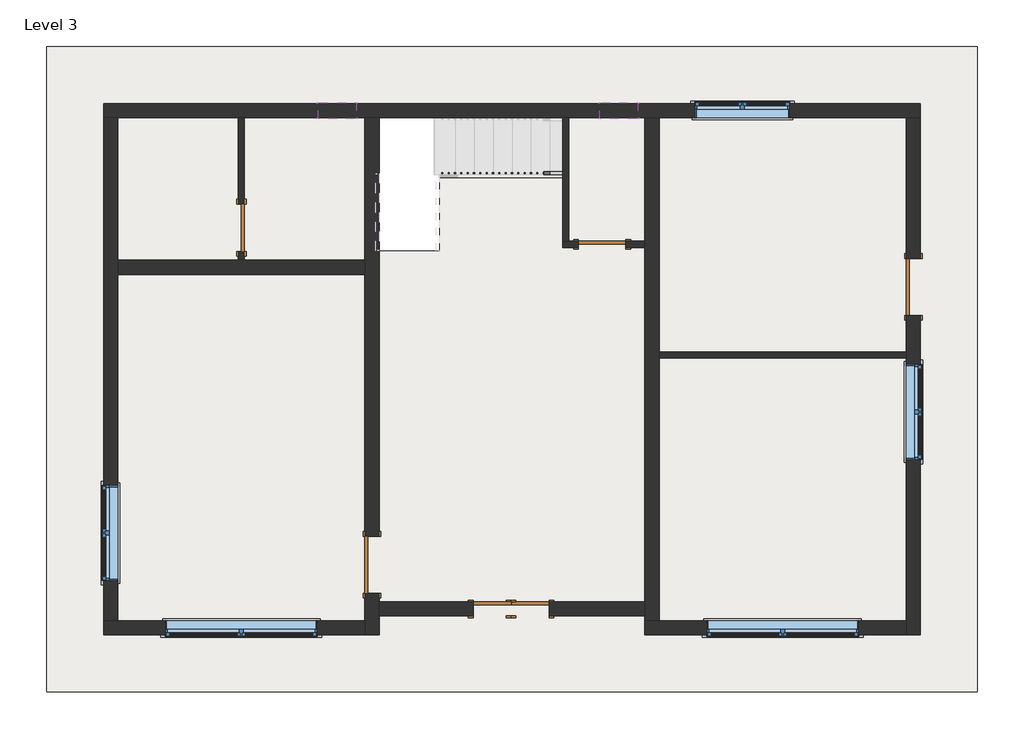
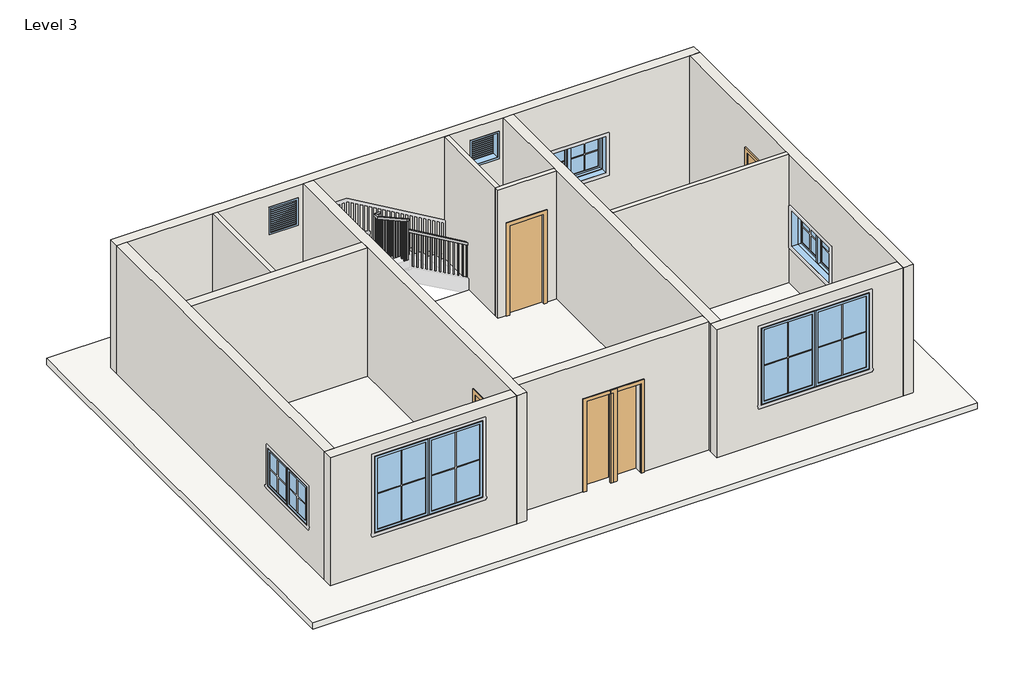
# One storey, part 1 of 2: 13 walls, 7 windows, 6 doors, 1 railing, 1 roof.
"""IFC4 building model written with IfcOpenShell, lengths in millimetres."""

from ifc_helpers import new_model, si_unit, frame, origin, place, context, project, spatial, polyline, outline, extrude, faceted_brep, transform, mapped, element, save
from components import single_flush_door_2_4a3212df, single_flush_door_2_0d3b4037, door_270f2424, door_aa9e95e7, single_flush_door_3_a90ba1ad, window_casement_double_c1d95f0f, window_casement_double_9ae172a2, window_f2d8fef0

model = new_model("IFC4")

# Units and contexts
model_context = context("Model", 3, world=origin())
ifc_project = project(units=[si_unit("LENGTHUNIT", "METRE", prefix="MILLI")], contexts=[model_context])

# Site, building, storey
site = spatial("IfcSite", under=ifc_project)
building = spatial("IfcBuilding", under=site)
storey = spatial("IfcBuildingStorey", under=building, Name="Level 3", Elevation=6248.4)

# Doors
placement = place(None, origin())
single_flush_door_2_shape = single_flush_door_2_4a3212df(model_context)
element("IfcDoor", 1, ObjectType="Single-Flush : DOOR 2'", at=placement, inside=storey, context=model_context, shape_type="MappedRepresentation", body=[
    mapped(single_flush_door_2_shape, transform((-1572.7415084, -2604.3618005, 6248.4), x_axis=(-1.0, 0.0, 0.0), y_axis=(0.0, -1.0, 0.0), z_axis=(0.0, 0.0, 1.0))),
])
single_flush_door_2_2_shape = single_flush_door_2_0d3b4037(model_context)
element("IfcDoor", 2, ObjectType="Single-Flush : DOOR 2'", at=placement, inside=storey, context=model_context, shape_type="MappedRepresentation", body=[
    mapped(single_flush_door_2_2_shape, transform((-963.1415084, -2604.3618005, 6248.4), x_axis=(1.0, 0.0, 0.0), y_axis=(0.0, 1.0, 0.0), z_axis=(0.0, 0.0, 1.0))),
])
door_shape = door_270f2424(model_context)
element("IfcDoor", 3, ObjectType="Single-Flush : DOOR 2'6\"", at=placement, inside=storey, context=model_context, shape_type="MappedRepresentation", body=[
    mapped(door_shape, transform((-5598.6415084, 3517.0381995, 6248.4), x_axis=(0.0, -1.0, 0.0), y_axis=(1.0, 0.0, 0.0), z_axis=(0.0, 0.0, 1.0))),
])
door_2_shape = door_aa9e95e7(model_context)
element("IfcDoor", 4, ObjectType="Single-Flush : DOOR 2'6\"", at=placement, inside=storey, context=model_context, shape_type="MappedRepresentation", body=[
    mapped(door_2_shape, transform((192.5584916, 3250.3381995, 6248.4), x_axis=(-1.0, 0.0, 0.0), y_axis=(0.0, -1.0, 0.0), z_axis=(0.0, 0.0, 1.0))),
])
single_flush_door_3_shape = single_flush_door_3_a90ba1ad(model_context)
element("IfcDoor", 5, ObjectType="Single-Flush : DOOR 3'", at=placement, inside=storey, context=model_context, shape_type="MappedRepresentation", body=[
    mapped(single_flush_door_3_shape, transform((-3503.1415084, -1893.1618005, 6248.4), x_axis=(0.0, -1.0, 0.0), y_axis=(1.0, 0.0, 0.0), z_axis=(0.0, 0.0, 1.0))),
])
element("IfcDoor", 6, ObjectType="Single-Flush : DOOR 3'", at=placement, inside=storey, context=model_context, shape_type="MappedRepresentation", body=[
    mapped(single_flush_door_3_shape, transform((5183.6584916, 2564.5381995, 6248.4), x_axis=(0.0, -1.0, 0.0), y_axis=(1.0, 0.0, 0.0), z_axis=(0.0, 0.0, 1.0))),
])

# Railing
element("IfcRailing", 7, ObjectType="Handrail - Rectangular", at=placement, inside=storey, context=model_context, shape_type="SolidModel", body=[
    faceted_brep([(-442.4415084, 4368.3146777, 7332.1333333), (-442.4415084, 4368.3146777, 7273.3219871), (-442.4415084, 4419.1146777, 7273.3219871), (-442.4415084, 4419.1146777, 7332.1333333), (-2398.2415084, 4368.3146777, 8473.0166667), (-2449.0415084, 4368.3146777, 8443.8386538), (-2449.0415084, 4419.1146777, 8443.8386538), (-2398.2415084, 4419.1146777, 8473.0166667), (-2398.2415084, 4368.3146777, 8729.1202697), (-2449.0415084, 4368.3146777, 8678.3202697), (-2449.0415084, 4419.1146777, 8678.3202697), (-2398.2415084, 4419.1146777, 8729.1202697), (-2474.4415084, 4368.3146777, 8729.1202697), (-2474.4415084, 4368.3146777, 8678.3202697), (-2525.2415084, 4419.1146777, 8678.3202697), (-2525.2415084, 4419.1146777, 8729.1202697), (-2474.4415084, 4292.1146777, 8729.1202697), (-2474.4415084, 4278.9546266, 8678.3202697), (-2525.2415084, 4278.9546266, 8678.3202697), (-2525.2415084, 4292.1146777, 8729.1202697), (-2474.4415084, 3148.7383287, 9364.1333333), (-2525.2415084, 3148.7383287, 9364.1333333), (-2525.2415084, 3148.7383287, 9306.02445), (-2474.4415084, 3148.7383287, 9306.02445)], [[[0, 1, 2, 3]], [[1, 0, 4, 5]], [[2, 1, 5, 6]], [[3, 2, 6, 7]], [[0, 3, 7, 4]], [[5, 4, 8, 9]], [[6, 5, 9, 10]], [[7, 6, 10, 11]], [[4, 7, 11, 8]], [[9, 8, 12, 13]], [[10, 9, 13, 14]], [[11, 10, 14, 15]], [[8, 11, 15, 12]], [[13, 12, 16, 17]], [[14, 13, 17, 18]], [[15, 14, 18, 19]], [[12, 15, 19, 16]], [[20, 21, 22, 23]], [[17, 16, 20, 23]], [[18, 17, 23, 22]], [[19, 18, 22, 21]], [[16, 19, 21, 20]]]),
    extrude(outline(polyline([(3184.0396777, 9286.5754052), (3184.0396777, 8280.4), (3164.9896777, 8280.4), (3164.9896777, 9297.1554726), (3184.0396777, 9286.5754052)])), frame((-2509.3665084, 0.0, 0.0), z_axis=(1.0, 0.0, 0.0), x_axis=(0.0, 1.0, 0.0)), (0.0, 0.0, 1.0), 19.05),
    extrude(outline(polyline([(3285.6396777, 9230.1483789), (3285.6396777, 8280.4), (3266.5896777, 8280.4), (3266.5896777, 9240.7284463), (3285.6396777, 9230.1483789)])), frame((-2509.3665084, 0.0, 0.0), z_axis=(1.0, 0.0, 0.0), x_axis=(0.0, 1.0, 0.0)), (0.0, 0.0, 1.0), 19.05),
    extrude(outline(polyline([(3387.2396777, 9173.7213526), (3387.2396777, 8280.4), (3368.1896777, 8280.4), (3368.1896777, 9184.3014201), (3387.2396777, 9173.7213526)])), frame((-2509.3665084, 0.0, 0.0), z_axis=(1.0, 0.0, 0.0), x_axis=(0.0, 1.0, 0.0)), (0.0, 0.0, 1.0), 19.05),
    extrude(outline(polyline([(3488.8396777, 9117.2420718), (3488.8396777, 8111.0666667), (3469.7896777, 8111.0666667), (3469.7896777, 9127.8221392), (3488.8396777, 9117.2420718)])), frame((-2509.3665084, 0.0, 0.0), z_axis=(1.0, 0.0, 0.0), x_axis=(0.0, 1.0, 0.0)), (0.0, 0.0, 1.0), 19.05),
    extrude(outline(polyline([(3590.4396777, 9060.8150456), (3590.4396777, 8111.0666667), (3571.3896777, 8111.0666667), (3571.3896777, 9071.395113), (3590.4396777, 9060.8150456)])), frame((-2509.3665084, 0.0, 0.0), z_axis=(1.0, 0.0, 0.0), x_axis=(0.0, 1.0, 0.0)), (0.0, 0.0, 1.0), 19.05),
    extrude(outline(polyline([(3692.0396777, 9004.3880193), (3692.0396777, 8111.0666667), (3672.9896777, 8111.0666667), (3672.9896777, 9014.9680867), (3692.0396777, 9004.3880193)])), frame((-2509.3665084, 0.0, 0.0), z_axis=(1.0, 0.0, 0.0), x_axis=(0.0, 1.0, 0.0)), (0.0, 0.0, 1.0), 19.05),
    extrude(outline(polyline([(3793.6396777, 8947.9087385), (3793.6396777, 7941.7333333), (3774.5896777, 7941.7333333), (3774.5896777, 8958.4888059), (3793.6396777, 8947.9087385)])), frame((-2509.3665084, 0.0, 0.0), z_axis=(1.0, 0.0, 0.0), x_axis=(0.0, 1.0, 0.0)), (0.0, 0.0, 1.0), 19.05),
    extrude(outline(polyline([(3895.2396777, 8891.4817122), (3895.2396777, 7941.7333333), (3876.1896777, 7941.7333333), (3876.1896777, 8902.0617797), (3895.2396777, 8891.4817122)])), frame((-2509.3665084, 0.0, 0.0), z_axis=(1.0, 0.0, 0.0), x_axis=(0.0, 1.0, 0.0)), (0.0, 0.0, 1.0), 19.05),
    extrude(outline(polyline([(3996.8396777, 8835.054686), (3996.8396777, 7941.7333333), (3977.7896777, 7941.7333333), (3977.7896777, 8845.6347534), (3996.8396777, 8835.054686)])), frame((-2509.3665084, 0.0, 0.0), z_axis=(1.0, 0.0, 0.0), x_axis=(0.0, 1.0, 0.0)), (0.0, 0.0, 1.0), 19.05),
    extrude(outline(polyline([(4098.4396777, 8778.5754052), (4098.4396777, 7772.4), (4079.3896777, 7772.4), (4079.3896777, 8789.1554726), (4098.4396777, 8778.5754052)])), frame((-2509.3665084, 0.0, 0.0), z_axis=(1.0, 0.0, 0.0), x_axis=(0.0, 1.0, 0.0)), (0.0, 0.0, 1.0), 19.05),
    extrude(outline(polyline([(4200.0396777, 8722.1483789), (4200.0396777, 7772.4), (4180.9896777, 7772.4), (4180.9896777, 8732.7284463), (4200.0396777, 8722.1483789)])), frame((-2509.3665084, 0.0, 0.0), z_axis=(1.0, 0.0, 0.0), x_axis=(0.0, 1.0, 0.0)), (0.0, 0.0, 1.0), 19.05),
    extrude(outline(polyline([(4301.6396777, 8665.7213526), (4301.6396777, 7772.4), (4282.5896777, 7772.4), (4282.5896777, 8676.3014201), (4301.6396777, 8665.7213526)])), frame((-2509.3665084, 0.0, 0.0), z_axis=(1.0, 0.0, 0.0), x_axis=(0.0, 1.0, 0.0)), (0.0, 0.0, 1.0), 19.05),
    extrude(outline(polyline([(-2464.9165084, 4384.1896777), (-2483.9665084, 4384.1896777), (-2483.9665084, 4403.2396777), (-2464.9165084, 4403.2396777), (-2464.9165084, 4384.1896777)])), frame((0.0, 0.0, 7603.0666667), z_axis=(0.0, 0.0, 1.0), x_axis=(1.0, 0.0, 0.0)), (0.0, 0.0, 1.0), 1075.253603),
    extrude(outline(polyline([(8404.9449038, -2382.3665084), (7433.7333333, -2382.3665084), (7433.7333333, -2363.3165084), (8393.8324038, -2363.3165084), (8404.9449038, -2382.3665084)])), frame((0.0, 4384.1896777, 0.0), z_axis=(0.0, 1.0, 0.0), x_axis=(0.0, 0.0, 1.0)), (0.0, 0.0, 1.0), 19.05),
    extrude(outline(polyline([(8345.6782371, -2280.7665084), (7433.7333333, -2280.7665084), (7433.7333333, -2261.7165084), (8334.5657371, -2261.7165084), (8345.6782371, -2280.7665084)])), frame((0.0, 4384.1896777, 0.0), z_axis=(0.0, 1.0, 0.0), x_axis=(0.0, 0.0, 1.0)), (0.0, 0.0, 1.0), 19.05),
    extrude(outline(polyline([(8286.4115704, -2179.1665084), (7433.7333333, -2179.1665084), (7433.7333333, -2160.1165084), (8275.2990704, -2160.1165084), (8286.4115704, -2179.1665084)])), frame((0.0, 4384.1896777, 0.0), z_axis=(0.0, 1.0, 0.0), x_axis=(0.0, 0.0, 1.0)), (0.0, 0.0, 1.0), 19.05),
    extrude(outline(polyline([(8227.1449038, -2077.5665084), (7264.4, -2077.5665084), (7264.4, -2058.5165084), (8216.0324038, -2058.5165084), (8227.1449038, -2077.5665084)])), frame((0.0, 4384.1896777, 0.0), z_axis=(0.0, 1.0, 0.0), x_axis=(0.0, 0.0, 1.0)), (0.0, 0.0, 1.0), 19.05),
    extrude(outline(polyline([(8167.8782371, -1975.9665084), (7264.4, -1975.9665084), (7264.4, -1956.9165084), (8156.7657371, -1956.9165084), (8167.8782371, -1975.9665084)])), frame((0.0, 4384.1896777, 0.0), z_axis=(0.0, 1.0, 0.0), x_axis=(0.0, 0.0, 1.0)), (0.0, 0.0, 1.0), 19.05),
    extrude(outline(polyline([(8108.6115704, -1874.3665084), (7264.4, -1874.3665084), (7264.4, -1855.3165084), (8097.4990704, -1855.3165084), (8108.6115704, -1874.3665084)])), frame((0.0, 4384.1896777, 0.0), z_axis=(0.0, 1.0, 0.0), x_axis=(0.0, 0.0, 1.0)), (0.0, 0.0, 1.0), 19.05),
    extrude(outline(polyline([(8049.3449038, -1772.7665084), (7095.0666667, -1772.7665084), (7095.0666667, -1753.7165084), (8038.2324038, -1753.7165084), (8049.3449038, -1772.7665084)])), frame((0.0, 4384.1896777, 0.0), z_axis=(0.0, 1.0, 0.0), x_axis=(0.0, 0.0, 1.0)), (0.0, 0.0, 1.0), 19.05),
    extrude(outline(polyline([(7990.0782371, -1671.1665084), (7095.0666667, -1671.1665084), (7095.0666667, -1652.1165084), (7978.9657371, -1652.1165084), (7990.0782371, -1671.1665084)])), frame((0.0, 4384.1896777, 0.0), z_axis=(0.0, 1.0, 0.0), x_axis=(0.0, 0.0, 1.0)), (0.0, 0.0, 1.0), 19.05),
    extrude(outline(polyline([(7930.8115704, -1569.5665084), (7095.0666667, -1569.5665084), (7095.0666667, -1550.5165084), (7919.6990704, -1550.5165084), (7930.8115704, -1569.5665084)])), frame((0.0, 4384.1896777, 0.0), z_axis=(0.0, 1.0, 0.0), x_axis=(0.0, 0.0, 1.0)), (0.0, 0.0, 1.0), 19.05),
    extrude(outline(polyline([(7871.5449038, -1467.9665084), (6925.7333333, -1467.9665084), (6925.7333333, -1448.9165084), (7860.4324038, -1448.9165084), (7871.5449038, -1467.9665084)])), frame((0.0, 4384.1896777, 0.0), z_axis=(0.0, 1.0, 0.0), x_axis=(0.0, 0.0, 1.0)), (0.0, 0.0, 1.0), 19.05),
    extrude(outline(polyline([(7812.2782371, -1366.3665084), (6925.7333333, -1366.3665084), (6925.7333333, -1347.3165084), (7801.1657371, -1347.3165084), (7812.2782371, -1366.3665084)])), frame((0.0, 4384.1896777, 0.0), z_axis=(0.0, 1.0, 0.0), x_axis=(0.0, 0.0, 1.0)), (0.0, 0.0, 1.0), 19.05),
    extrude(outline(polyline([(7753.0115704, -1264.7665084), (6925.7333333, -1264.7665084), (6925.7333333, -1245.7165084), (7741.8990704, -1245.7165084), (7753.0115704, -1264.7665084)])), frame((0.0, 4384.1896777, 0.0), z_axis=(0.0, 1.0, 0.0), x_axis=(0.0, 0.0, 1.0)), (0.0, 0.0, 1.0), 19.05),
    extrude(outline(polyline([(7693.7449038, -1163.1665084), (6756.4, -1163.1665084), (6756.4, -1144.1165084), (7682.6324038, -1144.1165084), (7693.7449038, -1163.1665084)])), frame((0.0, 4384.1896777, 0.0), z_axis=(0.0, 1.0, 0.0), x_axis=(0.0, 0.0, 1.0)), (0.0, 0.0, 1.0), 19.05),
    extrude(outline(polyline([(7634.4782371, -1061.5665084), (6756.4, -1061.5665084), (6756.4, -1042.5165084), (7623.3657371, -1042.5165084), (7634.4782371, -1061.5665084)])), frame((0.0, 4384.1896777, 0.0), z_axis=(0.0, 1.0, 0.0), x_axis=(0.0, 0.0, 1.0)), (0.0, 0.0, 1.0), 19.05),
    extrude(outline(polyline([(7575.2115704, -959.9665084), (6756.4, -959.9665084), (6756.4, -940.9165084), (7564.0990704, -940.9165084), (7575.2115704, -959.9665084)])), frame((0.0, 4384.1896777, 0.0), z_axis=(0.0, 1.0, 0.0), x_axis=(0.0, 0.0, 1.0)), (0.0, 0.0, 1.0), 19.05),
    extrude(outline(polyline([(7515.9449038, -858.3665084), (6587.0666667, -858.3665084), (6587.0666667, -839.3165084), (7504.8324038, -839.3165084), (7515.9449038, -858.3665084)])), frame((0.0, 4384.1896777, 0.0), z_axis=(0.0, 1.0, 0.0), x_axis=(0.0, 0.0, 1.0)), (0.0, 0.0, 1.0), 19.05),
    extrude(outline(polyline([(7456.6782371, -756.7665084), (6587.0666667, -756.7665084), (6587.0666667, -737.7165084), (7445.5657371, -737.7165084), (7456.6782371, -756.7665084)])), frame((0.0, 4384.1896777, 0.0), z_axis=(0.0, 1.0, 0.0), x_axis=(0.0, 0.0, 1.0)), (0.0, 0.0, 1.0), 19.05),
    extrude(outline(polyline([(7397.4115704, -655.1665084), (6587.0666667, -655.1665084), (6587.0666667, -636.1165084), (7386.2990704, -636.1165084), (7397.4115704, -655.1665084)])), frame((0.0, 4384.1896777, 0.0), z_axis=(0.0, 1.0, 0.0), x_axis=(0.0, 0.0, 1.0)), (0.0, 0.0, 1.0), 19.05),
    extrude(outline(polyline([(7338.1449038, -553.5665084), (6417.7333333, -553.5665084), (6417.7333333, -534.5165084), (7327.0324038, -534.5165084), (7338.1449038, -553.5665084)])), frame((0.0, 4384.1896777, 0.0), z_axis=(0.0, 1.0, 0.0), x_axis=(0.0, 0.0, 1.0)), (0.0, 0.0, 1.0), 19.05),
    extrude(outline(polyline([(-2490.3165084, 4384.1896777), (-2509.3665084, 4384.1896777), (-2509.3665084, 4403.2396777), (-2490.3165084, 4403.2396777), (-2490.3165084, 4384.1896777)])), frame((0.0, 0.0, 7603.0666667), z_axis=(0.0, 0.0, 1.0), x_axis=(1.0, 0.0, 0.0)), (0.0, 0.0, 1.0), 1075.253603),
    extrude(outline(polyline([(3167.7883287, 9295.4443826), (3167.7883287, 8280.4), (3148.7383287, 8280.4), (3148.7383287, 9306.02445), (3167.7883287, 9295.4443826)])), frame((-2509.3665084, 0.0, 0.0), z_axis=(1.0, 0.0, 0.0), x_axis=(0.0, 1.0, 0.0)), (0.0, 0.0, 1.0), 19.05),
    extrude(outline(polyline([(7284.4344871, -461.4915084), (6417.7333333, -461.4915084), (6417.7333333, -442.4415084), (7273.3219871, -442.4415084), (7284.4344871, -461.4915084)])), frame((0.0, 4384.1896777, 0.0), z_axis=(0.0, 1.0, 0.0), x_axis=(0.0, 0.0, 1.0)), (0.0, 0.0, 1.0), 19.05),
])

# Roof
element("IfcRoof", 8, ObjectType="ROOF 6\"", at=placement, inside=storey, context=model_context, shape_type="SweptSolid", body=[
    extrude(outline(polyline([(-8722.8415084, -3937.8618005), (-8722.8415084, 6425.3381995), (6212.3584916, 6425.3381995), (6212.3584916, -3937.8618005), (-8722.8415084, -3937.8618005)]), holes=[polyline([(-3439.6415084, 5333.1381995), (-3439.6415084, 3148.7383287), (-2423.6415084, 3148.7383287), (-2423.6415084, 4317.5146777), (-442.4415084, 4317.5146777), (-442.4415084, 5333.1381995), (-3439.6415084, 5333.1381995)])]), frame((0.0, 0.0, 6096.0), z_axis=(0.0, 0.0, 1.0), x_axis=(1.0, 0.0, 0.0)), (0.0, 0.0, 1.0), 152.4),
])

# Walls
element("IfcWall", 9, ObjectType="WALL 4\"", at=placement, inside=storey, context=model_context, shape_type="SweptSolid", body=[
    extrude(outline(polyline([(3136.0381995, 8382.0), (3136.0381995, 6248.4), (2996.3381995, 6248.4), (2996.3381995, 9296.4), (5282.3381995, 9296.4), (5282.3381995, 6248.4), (3898.0381995, 6248.4), (3898.0381995, 8382.0), (3136.0381995, 8382.0)])), frame((-5649.4415084, 0.0, 0.0), z_axis=(1.0, 0.0, 0.0), x_axis=(0.0, 1.0, 0.0)), (0.0, 0.0, 1.0), 101.6),
])
element("IfcWall", 10, ObjectType="WALL 4\"", at=placement, inside=storey, context=model_context, shape_type="Brep", body=[
    faceted_brep([(-188.4415084, 3301.1381995, 8382.0), (-188.4415084, 3301.1381995, 6248.4), (-340.8415084, 3301.1381995, 6248.4), (-442.4415084, 3301.1381995, 6248.4), (-442.4415084, 3301.1381995, 9296.4), (-340.8415084, 3301.1381995, 9296.4), (878.3584916, 3301.1381995, 9296.4), (878.3584916, 3301.1381995, 6248.4), (573.5584916, 3301.1381995, 6248.4), (573.5584916, 3301.1381995, 8382.0), (-442.4415084, 3199.5381995, 6248.4), (-188.4415084, 3199.5381995, 6248.4), (-188.4415084, 3199.5381995, 8382.0), (573.5584916, 3199.5381995, 8382.0), (573.5584916, 3199.5381995, 6248.4), (878.3584916, 3199.5381995, 6248.4), (878.3584916, 3199.5381995, 9296.4), (-442.4415084, 3199.5381995, 9296.4)], [[[0, 1, 2, 3, 4, 5, 6, 7, 8, 9]], [[10, 11, 12, 13, 14, 15, 16, 17]], [[8, 7, 15, 14]], [[3, 2, 1, 11, 10]], [[7, 6, 16, 15]], [[4, 3, 10, 17]], [[12, 11, 1, 0]], [[13, 12, 0, 9]], [[14, 13, 9, 8]], [[6, 5, 4, 17, 16]]]),
])
element("IfcWall", 11, ObjectType="WALL 4\"", at=placement, inside=storey, context=model_context, shape_type="Brep", body=[
    faceted_brep([(-340.8415084, 3301.1381995, 6248.4), (-340.8415084, 5282.3381995, 6248.4), (-340.8415084, 5282.3381995, 9296.4), (-340.8415084, 3301.1381995, 9296.4), (-442.4415084, 3301.1381995, 6248.4), (-442.4415084, 3301.1381995, 9296.4), (-442.4415084, 4317.5146777, 9296.4), (-442.4415084, 5282.3381995, 9296.4), (-442.4415084, 5282.3381995, 6248.4)], [[[0, 1, 2, 3]], [[4, 5, 6, 7, 8]], [[1, 0, 4, 8]], [[0, 3, 5, 4]], [[2, 1, 8, 7]], [[3, 2, 7, 6, 5]]]),
])
element("IfcWall", 12, ObjectType="WALL 4\"", at=placement, inside=storey, context=model_context, shape_type="SweptSolid", body=[
    extrude(outline(polyline([(1106.9584916, 1523.1381995), (5069.3584916, 1523.1381995), (5069.3584916, 1421.5381995), (1106.9584916, 1421.5381995), (1106.9584916, 1523.1381995)])), frame((0.0, 0.0, 6248.4), z_axis=(0.0, 0.0, 1.0), x_axis=(1.0, 0.0, 0.0)), (0.0, 0.0, 1.0), 3048.0),
])
element("IfcWall", 13, ObjectType="WALL 9\"", at=placement, inside=storey, context=model_context, shape_type="Brep", body=[
    faceted_brep([(-7808.4415084, 5282.3381995, 6248.4), (-7579.8415084, 5282.3381995, 6248.4), (-5649.4415084, 5282.3381995, 6248.4), (-5547.8415084, 5282.3381995, 6248.4), (-3617.4415084, 5282.3381995, 6248.4), (-3388.8415084, 5282.3381995, 6248.4), (-442.4415084, 5282.3381995, 6248.4), (-340.8415084, 5282.3381995, 6248.4), (878.3584916, 5282.3381995, 6248.4), (1106.9584916, 5282.3381995, 6248.4), (5069.3584916, 5282.3381995, 6248.4), (5297.9584916, 5282.3381995, 6248.4), (5297.9584916, 5282.3381995, 9296.4), (5069.3584916, 5282.3381995, 9296.4), (1106.9584916, 5282.3381995, 9296.4), (878.3584916, 5282.3381995, 9296.4), (-340.8415084, 5282.3381995, 9296.4), (-442.4415084, 5282.3381995, 9296.4), (-3388.8415084, 5282.3381995, 9296.4), (-3617.4415084, 5282.3381995, 9296.4), (-5547.8415084, 5282.3381995, 9296.4), (-5649.4415084, 5282.3381995, 9296.4), (-7579.8415084, 5282.3381995, 9296.4), (-7808.4415084, 5282.3381995, 9296.4), (3202.4584916, 5282.3381995, 8077.2), (3202.4584916, 5282.3381995, 7162.8), (1678.4584916, 5282.3381995, 7162.8), (1678.4584916, 5282.3381995, 8077.2), (154.4584916, 5282.3381995, 8991.6), (764.0584916, 5282.3381995, 8991.6), (764.0584916, 5282.3381995, 8382.0), (154.4584916, 5282.3381995, 8382.0), (-3757.1415084, 5282.3381995, 8991.6), (-3757.1415084, 5282.3381995, 8382.0), (-4366.7415084, 5282.3381995, 8382.0), (-4366.7415084, 5282.3381995, 8991.6), (-7808.4415084, 5510.9381995, 6248.4), (-7808.4415084, 5510.9381995, 9296.4), (5297.9584916, 5510.9381995, 9296.4), (5297.9584916, 5510.9381995, 6248.4), (3202.4584916, 5510.9381995, 8077.2), (1678.4584916, 5510.9381995, 8077.2), (1678.4584916, 5510.9381995, 7162.8), (3202.4584916, 5510.9381995, 7162.8), (154.4584916, 5510.9381995, 8991.6), (154.4584916, 5510.9381995, 8382.0), (764.0584916, 5510.9381995, 8382.0), (764.0584916, 5510.9381995, 8991.6), (-3757.1415084, 5510.9381995, 8991.6), (-4366.7415084, 5510.9381995, 8991.6), (-4366.7415084, 5510.9381995, 8382.0), (-3757.1415084, 5510.9381995, 8382.0)], [[[0, 1, 2, 3, 4, 5, 6, 7, 8, 9, 10, 11, 12, 13, 14, 15, 16, 17, 18, 19, 20, 21, 22, 23], [24, 25, 26, 27], [28, 29, 30, 31], [32, 33, 34, 35]], [[36, 37, 38, 39], [40, 41, 42, 43], [44, 45, 46, 47], [48, 49, 50, 51]], [[11, 10, 9, 8, 7, 6, 5, 4, 3, 2, 1, 0, 36, 39]], [[23, 22, 21, 20, 19, 18, 17, 16, 15, 14, 13, 12, 38, 37]], [[12, 11, 39, 38]], [[0, 23, 37, 36]], [[25, 24, 40, 43]], [[26, 25, 43, 42]], [[27, 26, 42, 41]], [[24, 27, 41, 40]], [[45, 44, 28, 31]], [[46, 45, 31, 30]], [[47, 46, 30, 29]], [[44, 47, 29, 28]], [[33, 32, 48, 51]], [[34, 33, 51, 50]], [[35, 34, 50, 49]], [[32, 35, 49, 48]]]),
])
element("IfcWall", 14, ObjectType="WALL 9\"", at=placement, inside=storey, context=model_context, shape_type="Brep", body=[
    faceted_brep([(5069.3584916, 2107.3381995, 8382.0), (5069.3584916, 2107.3381995, 6248.4), (5069.3584916, 1523.1381995, 6248.4), (5069.3584916, 1421.5381995, 6248.4), (5069.3584916, -2794.8618005, 6248.4), (5069.3584916, -3023.4618005, 6248.4), (5069.3584916, -3023.4618005, 9296.4), (5069.3584916, -2794.8618005, 9296.4), (5069.3584916, 1421.5381995, 9296.4), (5069.3584916, 1523.1381995, 9296.4), (5069.3584916, 5282.3381995, 9296.4), (5069.3584916, 5282.3381995, 6248.4), (5069.3584916, 3021.7381995, 6248.4), (5069.3584916, 3021.7381995, 8382.0), (5069.3584916, -204.0618005, 8077.2), (5069.3584916, -204.0618005, 7162.8), (5069.3584916, 1319.9381995, 7162.8), (5069.3584916, 1319.9381995, 8077.2), (5297.9584916, -3023.4618005, 6248.4), (5297.9584916, 2107.3381995, 6248.4), (5297.9584916, 2107.3381995, 8382.0), (5297.9584916, 3021.7381995, 8382.0), (5297.9584916, 3021.7381995, 6248.4), (5297.9584916, 5282.3381995, 6248.4), (5297.9584916, 5282.3381995, 9296.4), (5297.9584916, -3023.4618005, 9296.4), (5297.9584916, -204.0618005, 8077.2), (5297.9584916, 1319.9381995, 8077.2), (5297.9584916, 1319.9381995, 7162.8), (5297.9584916, -204.0618005, 7162.8)], [[[0, 1, 2, 3, 4, 5, 6, 7, 8, 9, 10, 11, 12, 13], [14, 15, 16, 17]], [[18, 19, 20, 21, 22, 23, 24, 25], [26, 27, 28, 29]], [[12, 11, 23, 22]], [[5, 4, 3, 2, 1, 19, 18]], [[11, 10, 24, 23]], [[6, 5, 18, 25]], [[15, 14, 26, 29]], [[16, 15, 29, 28]], [[17, 16, 28, 27]], [[14, 17, 27, 26]], [[20, 19, 1, 0]], [[21, 20, 0, 13]], [[22, 21, 13, 12]], [[10, 9, 8, 7, 6, 25, 24]]]),
])
element("IfcWall", 15, ObjectType="WALL 9\"", at=placement, inside=storey, context=model_context, shape_type="Brep", body=[
    faceted_brep([(5069.3584916, -2794.8618005, 6248.4), (1106.9584916, -2794.8618005, 6248.4), (878.3584916, -2794.8618005, 6248.4), (878.3584916, -2794.8618005, 9296.4), (1106.9584916, -2794.8618005, 9296.4), (5069.3584916, -2794.8618005, 9296.4), (1868.9584916, -2794.8618005, 8991.6), (1868.9584916, -2794.8618005, 7162.8), (4307.3584916, -2794.8618005, 7162.8), (4307.3584916, -2794.8618005, 8991.6), (5069.3584916, -3023.4618005, 6248.4), (5069.3584916, -3023.4618005, 9296.4), (878.3584916, -3023.4618005, 9296.4), (878.3584916, -3023.4618005, 6248.4), (1868.9584916, -3023.4618005, 8991.6), (4307.3584916, -3023.4618005, 8991.6), (4307.3584916, -3023.4618005, 7162.8), (1868.9584916, -3023.4618005, 7162.8)], [[[0, 1, 2, 3, 4, 5], [6, 7, 8, 9]], [[10, 11, 12, 13], [14, 15, 16, 17]], [[2, 1, 0, 10, 13]], [[0, 5, 11, 10]], [[3, 2, 13, 12]], [[7, 6, 14, 17]], [[8, 7, 17, 16]], [[9, 8, 16, 15]], [[6, 9, 15, 14]], [[5, 4, 3, 12, 11]]]),
])
element("IfcWall", 16, ObjectType="WALL 9\"", at=placement, inside=storey, context=model_context, shape_type="Brep", body=[
    faceted_brep([(1106.9584916, -2794.8618005, 6248.4), (1106.9584916, 1421.5381995, 6248.4), (1106.9584916, 1523.1381995, 6248.4), (1106.9584916, 5282.3381995, 6248.4), (1106.9584916, 5282.3381995, 9296.4), (1106.9584916, 1523.1381995, 9296.4), (1106.9584916, 1421.5381995, 9296.4), (1106.9584916, -2794.8618005, 9296.4), (878.3584916, -2794.8618005, 6248.4), (878.3584916, -2794.8618005, 9296.4), (878.3584916, -2718.6618005, 9296.4), (878.3584916, -2490.0618005, 9296.4), (878.3584916, 3199.5381995, 9296.4), (878.3584916, 3301.1381995, 9296.4), (878.3584916, 5282.3381995, 9296.4), (878.3584916, 5282.3381995, 6248.4), (878.3584916, 3301.1381995, 6248.4), (878.3584916, 3199.5381995, 6248.4), (878.3584916, -2490.0618005, 6248.4), (878.3584916, -2718.6618005, 6248.4)], [[[0, 1, 2, 3, 4, 5, 6, 7]], [[8, 9, 10, 11, 12, 13, 14, 15, 16, 17, 18, 19]], [[3, 2, 1, 0, 8, 19, 18, 17, 16, 15]], [[0, 7, 9, 8]], [[4, 3, 15, 14]], [[7, 6, 5, 4, 14, 13, 12, 11, 10, 9]]]),
])
element("IfcWall", 17, ObjectType="WALL 9\"", at=placement, inside=storey, context=model_context, shape_type="SweptSolid", body=[
    extrude(outline(polyline([(6248.4, 878.3584916), (9296.4, 878.3584916), (9296.4, -3388.8415084), (6248.4, -3388.8415084), (6248.4, -1877.5415084), (8382.0, -1877.5415084), (8382.0, -658.3415084), (6248.4, -658.3415084), (6248.4, 878.3584916)])), frame((0.0, -2718.6618005, 0.0), z_axis=(0.0, 1.0, 0.0), x_axis=(0.0, 0.0, 1.0)), (0.0, 0.0, 1.0), 228.6),
])
element("IfcWall", 18, ObjectType="WALL 9\"", at=placement, inside=storey, context=model_context, shape_type="Brep", body=[
    faceted_brep([(-3388.8415084, -3023.4618005, 6248.4), (-3388.8415084, -2718.6618005, 6248.4), (-3388.8415084, -2490.0618005, 6248.4), (-3388.8415084, -2350.3618005, 6248.4), (-3388.8415084, -2350.3618005, 8382.0), (-3388.8415084, -1435.9618005, 8382.0), (-3388.8415084, -1435.9618005, 6248.4), (-3388.8415084, 5282.3381995, 6248.4), (-3388.8415084, 5282.3381995, 9296.4), (-3388.8415084, -2490.0618005, 9296.4), (-3388.8415084, -2718.6618005, 9296.4), (-3388.8415084, -3023.4618005, 9296.4), (-3617.4415084, -2350.3618005, 8382.0), (-3617.4415084, -2350.3618005, 6248.4), (-3617.4415084, -2794.8618005, 6248.4), (-3617.4415084, -3023.4618005, 6248.4), (-3617.4415084, -3023.4618005, 9296.4), (-3617.4415084, -2794.8618005, 9296.4), (-3617.4415084, 2767.7381995, 9296.4), (-3617.4415084, 2996.3381995, 9296.4), (-3617.4415084, 5282.3381995, 9296.4), (-3617.4415084, 5282.3381995, 6248.4), (-3617.4415084, 2996.3381995, 6248.4), (-3617.4415084, 2767.7381995, 6248.4), (-3617.4415084, -1435.9618005, 6248.4), (-3617.4415084, -1435.9618005, 8382.0)], [[[0, 1, 2, 3, 4, 5, 6, 7, 8, 9, 10, 11]], [[12, 13, 14, 15, 16, 17, 18, 19, 20, 21, 22, 23, 24, 25]], [[15, 14, 13, 3, 2, 1, 0]], [[24, 23, 22, 21, 7, 6]], [[11, 10, 9, 8, 20, 19, 18, 17, 16]], [[8, 7, 21, 20]], [[0, 11, 16, 15]], [[4, 3, 13, 12]], [[5, 4, 12, 25]], [[6, 5, 25, 24]]]),
])
element("IfcWall", 19, ObjectType="WALL 9\"", at=placement, inside=storey, context=model_context, shape_type="Brep", body=[
    faceted_brep([(-3617.4415084, -2794.8618005, 6248.4), (-7579.8415084, -2794.8618005, 6248.4), (-7808.4415084, -2794.8618005, 6248.4), (-7808.4415084, -2794.8618005, 9296.4), (-7579.8415084, -2794.8618005, 9296.4), (-3617.4415084, -2794.8618005, 9296.4), (-6817.8415084, -2794.8618005, 8991.6), (-6817.8415084, -2794.8618005, 7162.8), (-4379.4415084, -2794.8618005, 7162.8), (-4379.4415084, -2794.8618005, 8991.6), (-3617.4415084, -3023.4618005, 6248.4), (-3617.4415084, -3023.4618005, 9296.4), (-7808.4415084, -3023.4618005, 9296.4), (-7808.4415084, -3023.4618005, 6248.4), (-6817.8415084, -3023.4618005, 8991.6), (-4379.4415084, -3023.4618005, 8991.6), (-4379.4415084, -3023.4618005, 7162.8), (-6817.8415084, -3023.4618005, 7162.8)], [[[0, 1, 2, 3, 4, 5], [6, 7, 8, 9]], [[10, 11, 12, 13], [14, 15, 16, 17]], [[2, 1, 0, 10, 13]], [[0, 5, 11, 10]], [[3, 2, 13, 12]], [[7, 6, 14, 17]], [[8, 7, 17, 16]], [[9, 8, 16, 15]], [[6, 9, 15, 14]], [[5, 4, 3, 12, 11]]]),
])
element("IfcWall", 20, ObjectType="WALL 9\"", at=placement, inside=storey, context=model_context, shape_type="Brep", body=[
    faceted_brep([(-7579.8415084, -2794.8618005, 6248.4), (-7579.8415084, 2767.7381995, 6248.4), (-7579.8415084, 2996.3381995, 6248.4), (-7579.8415084, 5282.3381995, 6248.4), (-7579.8415084, 5282.3381995, 9296.4), (-7579.8415084, 2996.3381995, 9296.4), (-7579.8415084, 2767.7381995, 9296.4), (-7579.8415084, -2794.8618005, 9296.4), (-7579.8415084, -623.1618005, 8077.2), (-7579.8415084, -623.1618005, 7162.8), (-7579.8415084, -2147.1618005, 7162.8), (-7579.8415084, -2147.1618005, 8077.2), (-7808.4415084, -2794.8618005, 6248.4), (-7808.4415084, -2794.8618005, 9296.4), (-7808.4415084, 5282.3381995, 9296.4), (-7808.4415084, 5282.3381995, 6248.4), (-7808.4415084, -623.1618005, 8077.2), (-7808.4415084, -2147.1618005, 8077.2), (-7808.4415084, -2147.1618005, 7162.8), (-7808.4415084, -623.1618005, 7162.8)], [[[0, 1, 2, 3, 4, 5, 6, 7], [8, 9, 10, 11]], [[12, 13, 14, 15], [16, 17, 18, 19]], [[3, 2, 1, 0, 12, 15]], [[0, 7, 13, 12]], [[4, 3, 15, 14]], [[9, 8, 16, 19]], [[10, 9, 19, 18]], [[11, 10, 18, 17]], [[8, 11, 17, 16]], [[7, 6, 5, 4, 14, 13]]]),
])
element("IfcWall", 21, ObjectType="WALL 9\"", at=placement, inside=storey, context=model_context, shape_type="Brep", body=[
    faceted_brep([(-7579.8415084, 2767.7381995, 6248.4), (-3617.4415084, 2767.7381995, 6248.4), (-3617.4415084, 2767.7381995, 9296.4), (-7579.8415084, 2767.7381995, 9296.4), (-7579.8415084, 2996.3381995, 6248.4), (-7579.8415084, 2996.3381995, 9296.4), (-5649.4415084, 2996.3381995, 9296.4), (-5547.8415084, 2996.3381995, 9296.4), (-3617.4415084, 2996.3381995, 9296.4), (-3617.4415084, 2996.3381995, 6248.4), (-5547.8415084, 2996.3381995, 6248.4), (-5649.4415084, 2996.3381995, 6248.4)], [[[0, 1, 2, 3]], [[4, 5, 6, 7, 8, 9, 10, 11]], [[1, 0, 4, 11, 10, 9]], [[2, 1, 9, 8]], [[0, 3, 5, 4]], [[3, 2, 8, 7, 6, 5]]]),
])

# Windows
window_casement_double_shape = window_casement_double_c1d95f0f(model_context)
element("IfcWindow", 22, ObjectType="Window-Casement-Double", at=placement, inside=storey, context=model_context, shape_type="MappedRepresentation", body=[
    mapped(window_casement_double_shape, transform((-7694.1415084, -1385.1618005, 6248.4), x_axis=(0.0, 1.0, 0.0), y_axis=(-1.0, 0.0, 0.0), z_axis=(0.0, 0.0, 1.0))),
])
element("IfcWindow", 23, ObjectType="Window-Casement-Double", at=placement, inside=storey, context=model_context, shape_type="MappedRepresentation", body=[
    mapped(window_casement_double_shape, transform((5183.6584916, 557.9381995, 6248.4), x_axis=(0.0, -1.0, 0.0), y_axis=(1.0, 0.0, 0.0), z_axis=(0.0, 0.0, 1.0))),
])
element("IfcWindow", 24, ObjectType="Window-Casement-Double", at=placement, inside=storey, context=model_context, shape_type="MappedRepresentation", body=[
    mapped(window_casement_double_shape, transform((2440.4584916, 5396.6381995, 6248.4), x_axis=(1.0, 0.0, 0.0), y_axis=(0.0, 1.0, 0.0), z_axis=(0.0, 0.0, 1.0))),
])
window_casement_double_2_shape = window_casement_double_9ae172a2(model_context)
element("IfcWindow", 25, ObjectType="Window-Casement-Double", at=placement, inside=storey, context=model_context, shape_type="MappedRepresentation", body=[
    mapped(window_casement_double_2_shape, transform((-5598.6415084, -2909.1618005, 6248.4), x_axis=(-1.0, 0.0, 0.0), y_axis=(0.0, -1.0, 0.0), z_axis=(0.0, 0.0, 1.0))),
])
element("IfcWindow", 26, ObjectType="Window-Casement-Double", at=placement, inside=storey, context=model_context, shape_type="MappedRepresentation", body=[
    mapped(window_casement_double_2_shape, transform((3088.1584916, -2909.1618005, 6248.4), x_axis=(-1.0, 0.0, 0.0), y_axis=(0.0, -1.0, 0.0), z_axis=(0.0, 0.0, 1.0))),
])
window_shape = window_f2d8fef0(model_context)
element("IfcWindow", 27, ObjectType="Window-Louvers : 24\" x 24\"", at=placement, inside=storey, context=model_context, shape_type="MappedRepresentation", body=[
    mapped(window_shape, transform((459.2584916, 5402.9881995, 7467.6), x_axis=(1.0, 0.0, 0.0), y_axis=(0.0, 1.0, 0.0), z_axis=(0.0, 0.0, 1.0))),
])
element("IfcWindow", 28, ObjectType="Window-Louvers : 24\" x 24\"", at=placement, inside=storey, context=model_context, shape_type="MappedRepresentation", body=[
    mapped(window_shape, transform((-4061.9415084, 5390.2881995, 7467.6), x_axis=(-1.0, 0.0, 0.0), y_axis=(0.0, -1.0, 0.0), z_axis=(0.0, 0.0, 1.0))),
])

save(model, "model.ifc")

# Revit data of these elements
# Type "Single-Flush : DOOR 2'"
#   Type Mark = "10"
#   Construction Type Id = "MDOOR"
#   Assembly Code = "C1020"
#   Analytic Construction = "Metal"
#   Thickness = 0' - 2"
#   Heat Transfer Coefficient (U) = 0.651978 BTU/(h·ft²·°F)
#   Height = 7' - 0"
#   Trim Projection Ext = 0' - 1"
#   Trim Projection Int = 0' - 1"
#   Trim Width = 0' - 3"
#   Width = 2' - 0"
#   Define Thermal Properties by = 1
#   Door Material = Door - Panel
#   Frame Material = Door - Frame
#   Visual Light Transmittance = 0
#   Solar Heat Gain Coefficient = 0
#   Function = (empty or 0)
#   Wall Closure = (empty or 0)
# Type "Single-Flush : DOOR 2'6\""
#   Type Mark = "9"
#   Construction Type Id = "MDOOR"
#   Assembly Code = "C1020"
#   Analytic Construction = "Metal"
#   Thickness = 0' - 2"
#   Heat Transfer Coefficient (U) = 0.651978 BTU/(h·ft²·°F)
#   Height = 7' - 0"
#   Trim Projection Ext = 0' - 1"
#   Trim Projection Int = 0' - 1"
#   Trim Width = 0' - 3"
#   Width = 2' - 6"
#   Define Thermal Properties by = 1
#   Door Material = Door - Panel
#   Frame Material = Door - Frame
#   Visual Light Transmittance = 0
#   Solar Heat Gain Coefficient = 0
#   Function = (empty or 0)
#   Wall Closure = (empty or 0)
# Type "Single-Flush : DOOR 3'"
#   Type Mark = "8"
#   Construction Type Id = "MDOOR"
#   Assembly Code = "C1020"
#   Analytic Construction = "Metal"
#   Thickness = 0' - 2"
#   Heat Transfer Coefficient (U) = 0.651978 BTU/(h·ft²·°F)
#   Height = 7' - 0"
#   Trim Projection Ext = 0' - 1"
#   Trim Projection Int = 0' - 1"
#   Trim Width = 0' - 3"
#   Width = 3' - 0"
#   Define Thermal Properties by = 1
#   Door Material = Door - Panel
#   Frame Material = Door - Frame
#   Visual Light Transmittance = 0
#   Solar Heat Gain Coefficient = 0
#   Function = (empty or 0)
#   Wall Closure = (empty or 0)
# Type "Handrail - Rectangular"
#   Assembly Code = "C2010400"
#   built-in parameter 1008612 = 0.0416667 (stored number, unit not read)
#   built-in parameter 1008611 = 0.0416667 (stored number, unit not read)
#   built-in parameter 1008609 = 0.333333 (stored number, unit not read)
#   built-in parameter 1008604 = 0.166667 (stored number, unit not read)
#   built-in parameter 1008603 = 0.166667 (stored number, unit not read)
#   Railing Height = 3' - 0"
#   built-in parameter 1008630 = 2
#   built-in parameter 1008610 = 2
#   built-in parameter 1008618 = Baluster - Square : 3/4"
# Type "ROOF 6\""
#   Assembly Code = "B1020"
#   Layers, outside or top first: 0' - 6" no material (function 1)
# Type "WALL 4\""
#   Assembly Code = "B2010"
#   Layers, outside or top first: 0' - 4" no material (function 1)
# Type "WALL 9\""
#   Assembly Code = "B2010"
#   Layers, outside or top first: 0' - 9" no material (function 1)
# Type "Window-Casement-Double"
#   Type Mark = "18"
#   Fire Rating = "0.5h"
#   Assembly Code = "B2020100"
#   Analytic Construction = "Double glazing - domestic"
#   Frame Extension [instance default] = 0' - 0 1/4"
#   Window Inset [instance default] = 0' - 0"
#   Wall Thickness [instance default] = 0' - 6"
#   Interior Wall Closure [instance default] = 0' - 2 1/4"
#   Half Width = 2' - 6"
#   Visual Light Transmittance = 0.81
#   Thermal Resistance (R) = 1.8146 (h·ft²·°F)/BTU
#   Solar Heat Gain Coefficient = 0.76
#   Rough Width = 5' - 0 1/2"
#   Rough Height = 3' - 0 1/2"
#   Height = 3' - 0"
#   Heat Transfer Coefficient (U) = 0.5511 BTU/(h·ft²·°F)
#   Exterior Wall Closure [instance default] = 0' - 1 1/4"
#   Extension Jamb [instance default] = 0' - 2 1/4"
#   Default Sill Height = 3' - 0"
#   Width = 5' - 0"
#   Muntin Visibility = yes
#   Interior Trim Visibility [instance default] = yes
#   Exterior Trim Visibility [instance default] = yes
#   Extension Jamb Visibility [instance default] = yes
#   Interior Trim Material = Wood - Stained
#   Muntin Pattern = Muntin Pattern_2x2 : Muntin Pattern_2x2
#   Interior Trim = Trim-Window-Interior-Flat : Picture Frame
#   Interior Frame Material = Wood - Stained
#   Glass Panel Material = Glass
#   Exterior Trim Material = Clad - White
#   Exterior Trim = Trim-Window-Exterior-Flat : with Sill
#   Exterior Frame Material = Clad - White
#   Wall Closure = (empty or 0)
# Type "Window-Casement-Double"
#   Type Mark = "19"
#   Fire Rating = "0.5h"
#   Assembly Code = "B2020100"
#   Analytic Construction = "Double glazing - domestic"
#   Frame Extension [instance default] = 0' - 0 1/4"
#   Window Inset [instance default] = 0' - 0"
#   Wall Thickness [instance default] = 0' - 6"
#   Interior Wall Closure [instance default] = 0' - 2 1/4"
#   Half Width = 4' - 0"
#   Visual Light Transmittance = 0.81
#   Thermal Resistance (R) = 1.8146 (h·ft²·°F)/BTU
#   Solar Heat Gain Coefficient = 0.76
#   Rough Width = 8' - 0 1/2"
#   Rough Height = 6' - 0 1/2"
#   Height = 6' - 0"
#   Heat Transfer Coefficient (U) = 0.5511 BTU/(h·ft²·°F)
#   Exterior Wall Closure [instance default] = 0' - 1 1/4"
#   Extension Jamb [instance default] = 0' - 2 1/4"
#   Default Sill Height = 3' - 0"
#   Width = 8' - 0"
#   Muntin Visibility = yes
#   Interior Trim Visibility [instance default] = yes
#   Exterior Trim Visibility [instance default] = yes
#   Extension Jamb Visibility [instance default] = yes
#   Interior Trim Material = Wood - Stained
#   Muntin Pattern = Muntin Pattern_2x2 : Muntin Pattern_2x2
#   Interior Trim = Trim-Window-Interior-Flat : Picture Frame
#   Interior Frame Material = Wood - Stained
#   Glass Panel Material = Glass
#   Exterior Trim Material = Clad - White
#   Exterior Trim = Trim-Window-Exterior-Flat : with Sill
#   Exterior Frame Material = Clad - White
#   Wall Closure = (empty or 0)
# Type "Window-Louvers : 24\" x 24\""
#   Type Mark = "20"
#   Construction Type Id = "GSP4R"
#   Assembly Code = "B20"
#   Analytic Construction = "1/8 in Pilkington single glazing"
#   Visual Light Transmittance = 0.9
#   Thermal Resistance (R) = 1.53941 (h·ft²·°F)/BTU
#   Solar Heat Gain Coefficient = 0.78
#   Max Height = 1' - 11.74264"
#   Height = 2' - 0"
#   Heat Transfer Coefficient (U) = 0.6496 BTU/(h·ft²·°F)
#   Blade Width [instance default] = 1' - 10 1/2"
#   Blade Vertical Thickness = 0' - 0.35355"
#   Blade Thickness = 0' - 0 1/4"
#   Blade Spacing = 0' - 1 1/2"
#   Blade Height = 0' - 1.85355"
#   Blade Depth = 0' - 3"
#   Blade Angle = 45.00°
#   Default Sill Height = 3' - 0"
#   Trim Projection_Exterior = 0' - 0 1/2"
#   Trim Projection_Interior = 0' - 0 1/2"
#   Trim Width_Exterior = 0' - 1 1/2"
#   Trim Width_Interior = 0' - 1 1/2"
#   Width = 2' - 0"
#   Max Blade Count = 12
#   Define Thermal Properties by = 1
#   Blade Count = 12
#   Frame Material = Birch
#   Louver Material = Birch
#   Trim Exterior Material = Birch
#   Trim Interior Material = Birch
#   Wall Closure = (empty or 0)
# Elements 1, 2 (IfcDoor, "Single-Flush : DOOR 2'")
#   Phase Created = New Construction
#   Materials on its faces: "Door - Frame", "Door - Panel"
# Elements 3, 4 (IfcDoor, "Single-Flush : DOOR 2'6\"")
#   Phase Created = New Construction
#   Materials on its faces: "Door - Frame", "Door - Panel"
# Elements 5, 6 (IfcDoor, "Single-Flush : DOOR 3'")
#   Phase Created = New Construction
#   Materials on its faces: "Door - Frame", "Door - Panel"
# Element 7 (IfcRailing, "Handrail - Rectangular")
#   Phase Created = New Construction
# Element 8 (IfcRoof, "ROOF 6\"")
#   built-in parameter 1001705 = 20.5 (stored number, unit not read)
#   built-in parameter 1001701 = -0.5 (stored number, unit not read)
#   built-in parameter 1001710 = 33615
#   Phase Created = New Construction
#   Materials on its faces: "Door - Frame", "Default Roof", "Wood - Stained"
# Elements 9, 12 (IfcWall, "WALL 4\"")
#   Top Offset = 0' - 0"
#   Base Offset = 0' - 0"
#   Unconnected Height = 10' - 0"
#   wall height = 10' - 0"
#   Phase Created = New Construction
#   Base Constraint = Level 3
#   Materials on its faces: "Default Wall"
# Elements 10, 11 (IfcWall, "WALL 4\"")
#   Top Offset = 0' - 0"
#   Base Offset = 0' - 0"
#   Unconnected Height = 10' - 0"
#   wall height = 10' - 0"
#   Phase Created = New Construction
#   Base Constraint = Level 3
#   Materials on its faces: "Default Wall", "Door - Frame"
# Element 13 (IfcWall, "WALL 9\"")
#   Top Offset = 0' - 0"
#   Base Offset = 0' - 0"
#   Unconnected Height = 10' - 0"
#   wall height = 10' - 0"
#   Phase Created = New Construction
#   Base Constraint = Level 3
#   Materials on its faces: "Default Wall", "Parking Stripe", "Door - Frame"
# Elements 14, 15, 16, 17, 19, 20 (IfcWall, "WALL 9\"")
#   Top Offset = 0' - 0"
#   Base Offset = 0' - 0"
#   Unconnected Height = 10' - 0"
#   wall height = 10' - 0"
#   Phase Created = New Construction
#   Base Constraint = Level 3
#   Materials on its faces: "Default Wall", "Parking Stripe"
# Element 18 (IfcWall, "WALL 9\"")
#   Top Offset = 0' - 0"
#   Base Offset = 0' - 0"
#   Unconnected Height = 10' - 0"
#   wall height = 10' - 0"
#   Phase Created = New Construction
#   Base Constraint = Level 3
#   Materials on its faces: "Default Wall", "Door - Frame", "Parking Stripe"
# Element 21 (IfcWall, "WALL 9\"")
#   Top Offset = 0' - 0"
#   Base Offset = 0' - 0"
#   Unconnected Height = 10' - 0"
#   wall height = 10' - 0"
#   Phase Created = New Construction
#   Base Constraint = Level 3
#   Materials on its faces: "Default Wall"
# Element 22 (IfcWindow, "Window-Casement-Double")
#   Mark = "15"
#   Window Inset = 0' - 0"
#   Interior Wall Closure = 0' - 2 1/4"
#   Frame Extension = 0' - 0 1/4"
#   Exterior Wall Closure = 0' - 1 1/4"
#   Interior Trim Visibility = yes
#   Exterior Trim Visibility = yes
#   Phase Created = New Construction
#   Materials on its faces: "Wood - Stained", "Glass", "Clad - White"
# Element 23 (IfcWindow, "Window-Casement-Double")
#   Mark = "16"
#   Window Inset = 0' - 0"
#   Interior Wall Closure = 0' - 2 1/4"
#   Frame Extension = 0' - 0 1/4"
#   Exterior Wall Closure = 0' - 1 1/4"
#   Interior Trim Visibility = yes
#   Exterior Trim Visibility = yes
#   Phase Created = New Construction
#   Materials on its faces: "Wood - Stained", "Glass", "Clad - White"
# Element 24 (IfcWindow, "Window-Casement-Double")
#   Mark = "17"
#   Window Inset = 0' - 0"
#   Interior Wall Closure = 0' - 2 1/4"
#   Frame Extension = 0' - 0 1/4"
#   Exterior Wall Closure = 0' - 1 1/4"
#   Interior Trim Visibility = yes
#   Exterior Trim Visibility = yes
#   Phase Created = New Construction
#   Materials on its faces: "Wood - Stained", "Glass", "Clad - White"
# Element 25 (IfcWindow, "Window-Casement-Double")
#   Mark = "18"
#   Window Inset = 0' - 0"
#   Interior Wall Closure = 0' - 2 1/4"
#   Frame Extension = 0' - 0 1/4"
#   Exterior Wall Closure = 0' - 1 1/4"
#   Interior Trim Visibility = yes
#   Exterior Trim Visibility = yes
#   Phase Created = New Construction
#   Materials on its faces: "Wood - Stained", "Glass", "Clad - White"
# Element 26 (IfcWindow, "Window-Casement-Double")
#   Mark = "19"
#   Window Inset = 0' - 0"
#   Interior Wall Closure = 0' - 2 1/4"
#   Frame Extension = 0' - 0 1/4"
#   Exterior Wall Closure = 0' - 1 1/4"
#   Interior Trim Visibility = yes
#   Exterior Trim Visibility = yes
#   Phase Created = New Construction
#   Materials on its faces: "Wood - Stained", "Glass", "Clad - White"
# Element 27 (IfcWindow, "Window-Louvers : 24\" x 24\"")
#   Mark = "20"
#   Blade Width = 1' - 10 1/2"
#   Phase Created = New Construction
#   Materials on its faces: "Birch"
# Element 28 (IfcWindow, "Window-Louvers : 24\" x 24\"")
#   Mark = "21"
#   Blade Width = 1' - 10 1/2"
#   Phase Created = New Construction
#   Materials on its faces: "Birch"
# Materials
#   "Door - Panel": class "Wood", colour RGB 210 159 95, transparency 0, Cost = 0
#   "Door - Frame": colour RGB 118 70 51, transparency 0, Cost = 0
#   "Wood - Stained": class "Wood", colour RGB 224 178 126, transparency 0, Cost = 0
#   "Glass": class "Glass", colour RGB 0 128 192, transparency 0.75, Description = "Soda Lime Glass", Cost = 0
#   "Clad - White": class "Wood", colour RGB 242 242 238, transparency 0, Cost = 0
#   "Birch": class "Wood", colour RGB 224 178 126, transparency 0, Description = "Betula Alleghaniensis", Cost = 0
#   "Default Roof": colour RGB 88 101 114, transparency 0, Cost = 0
#   "Default Wall": colour RGB 128 128 128, transparency 0, Cost = 0
#   "Parking Stripe": class "Paint", colour RGB 250 250 91, transparency 0, Cost = 0
